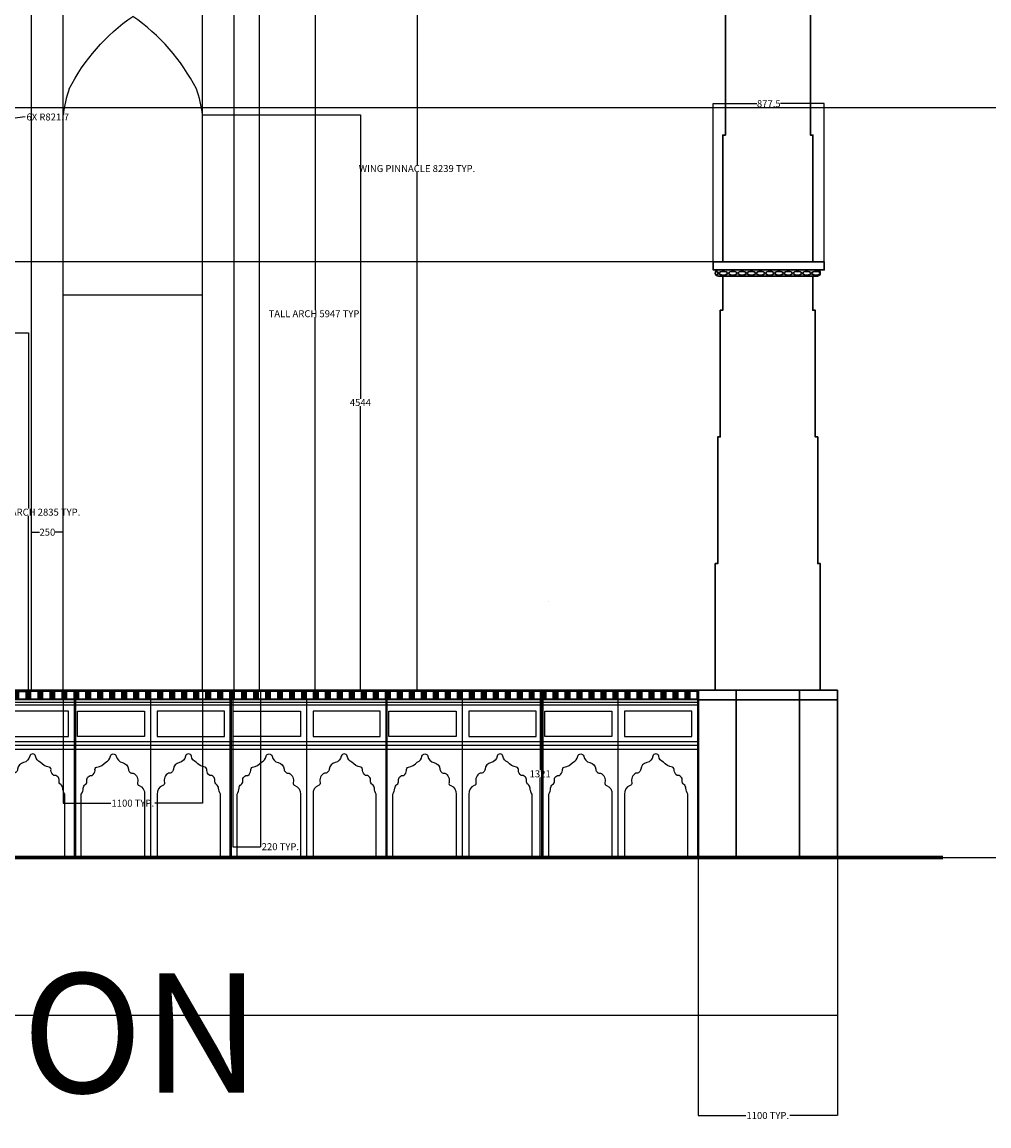
# Model space of a CAD drawing. Units: millimetres. Extents: x 8570 to 49085, y 3782 to 24863.
# Tile 8 of 15: x 27529 to 35169, y 3782 to 12499. Entities that reach past the tile are written whole.
import ezdxf

# ---------------------------------------------------------------- set-up
doc = ezdxf.new("R2010")
doc.units = ezdxf.units.MM
doc.header["$MEASUREMENT"] = 0
doc.header["$PDMODE"] = 3
for name, color, linetype, lineweight in [('A-ANNO-DIMS', 2, 'Continuous', 18), ('A-ANNO-TEXT', 7, 'Continuous', 25), ('A-ELEV-ARCH', 7, 'Continuous', 25), ('A-ELEV-GRND', 7, 'Continuous', 35), ('A-ELEV-MNRT', 7, 'Continuous', 30), ('A-ELEV-PATT', 252, 'Continuous', 13), ('A-ELEV-PIER', 7, 'Continuous', 25), ('A-ELEV-PLIN', 7, 'Continuous', 25)]:
    doc.layers.add(name, color=color, linetype=linetype, lineweight=lineweight)
doc.styles.get("Standard").update_dxf_attribs({"font": 'arial.ttf'})
doc.dimstyles.get("Standard").update_dxf_attribs({"dimtxt": 55, "dimasz": 0.18, "dimexe": 0.18, "dimexo": 0.0625, "dimgap": 0.09, "dimtad": 0, "dimtih": 1, "dimtoh": 1, "dimdec": 0, "dimzin": 0, "dimdsep": 46, "dimtxsty": 'Standard', "dimcen": 0.09, "dimadec": 0, "dimazin": 0, "dimtfac": 1, "dimtdec": 0, "dimtofl": 0, "dimtmove": 0, "dimatfit": 3, "dimfxl": 1, "dimtolj": 1, "dimtzin": 0, "dimarcsym": 0})

# ---------------------------------------------------------------- blocks, each defined once
blk = doc.blocks.new('MINARET-ELEV')
h = blk.add_hatch(color=256)
h.dxf.hatch_style = 1
edge = h.paths.add_edge_path()
edge.add_arc((788.1, 7879), 96, 347.52389, 357.31225, ccw=False)
edge.add_ellipse((859.2, 7847.7), major_axis=(31.8, 0), ratio=0.472441, start_angle=385.01443, end_angle=315.51296)
edge.add_arc((788.1, 7879), 96, 325.26025, 332.17741, ccw=False)
edge.add_line((867, 7824.3), (235, 7824.3))
edge.add_arc((313.9, 7879), 96, 182.68775, 214.73975, ccw=False)
edge.add_line((218, 7874.5), (884, 7874.5))
edge = h.paths.add_edge_path(flags=16)
edge.add_ellipse((494.2, 7847.7), major_axis=(31.8, 0), ratio=0.472441, start_angle=0, end_angle=360, ccw=False)
edge = h.paths.add_edge_path(flags=16)
edge.add_ellipse((567.2, 7847.7), major_axis=(31.8, 0), ratio=0.472441, start_angle=0, end_angle=360, ccw=False)
edge = h.paths.add_edge_path(flags=16)
edge.add_ellipse((421.2, 7847.7), major_axis=(31.8, 0), ratio=0.472441, start_angle=0, end_angle=360, ccw=False)
edge = h.paths.add_edge_path(flags=16)
edge.add_ellipse((640.2, 7847.7), major_axis=(31.8, 0), ratio=0.472441, start_angle=0, end_angle=360, ccw=False)
edge = h.paths.add_edge_path(flags=16)
edge.add_ellipse((348.2, 7847.7), major_axis=(31.8, 0), ratio=0.472441, start_angle=0, end_angle=360, ccw=False)
edge = h.paths.add_edge_path(flags=16)
edge.add_ellipse((713.2, 7847.7), major_axis=(31.8, 0), ratio=0.472441, start_angle=0, end_angle=360, ccw=False)
edge = h.paths.add_edge_path(flags=16)
edge.add_ellipse((275.2, 7847.7), major_axis=(31.8, 0), ratio=0.472441, start_angle=0, end_angle=360, ccw=False)
edge = h.paths.add_edge_path(flags=16)
edge.add_ellipse((786.2, 7847.7), major_axis=(31.8, 0), ratio=0.472441, start_angle=0, end_angle=360, ccw=False)
h = blk.add_hatch(color=256)
h.dxf.hatch_style = 1
edge = h.paths.add_edge_path()
edge.add_arc((940, 4615.3), 25, 270, 450, ccw=False)
edge.add_line((940, 4590.3), (160, 4590.3))
edge.add_arc((160, 4615.3), 25, 217.6761, 270, ccw=False)
edge.add_ellipse((127.2, 4613.7), major_axis=(31.8, 0), ratio=0.472441, start_angle=313.43175, end_angle=411.74889)
edge.add_arc((160, 4615.3), 25, 450, 510.08055, ccw=False)
edge.add_line((160, 4640.3), (940, 4640.3))
edge = h.paths.add_edge_path(flags=16)
edge.add_ellipse((347.2, 4613.7), major_axis=(31.8, 0), ratio=0.472441, start_angle=0, end_angle=360, ccw=False)
edge = h.paths.add_edge_path(flags=16)
edge.add_ellipse((420.2, 4613.7), major_axis=(31.8, 0), ratio=0.472441, start_angle=0, end_angle=360, ccw=False)
edge = h.paths.add_edge_path(flags=16)
edge.add_ellipse((274.2, 4613.7), major_axis=(31.8, 0), ratio=0.472441, start_angle=0, end_angle=360, ccw=False)
edge = h.paths.add_edge_path(flags=16)
edge.add_ellipse((493.2, 4613.7), major_axis=(31.8, 0), ratio=0.472441, start_angle=0, end_angle=360, ccw=False)
edge = h.paths.add_edge_path(flags=16)
edge.add_ellipse((198.8, 4613.7), major_axis=(31.8, 0), ratio=0.472441, start_angle=0, end_angle=360, ccw=False)
edge = h.paths.add_edge_path(flags=16)
edge.add_ellipse((566.2, 4613.7), major_axis=(31.8, 0), ratio=0.472441, start_angle=0, end_angle=360, ccw=False)
edge = h.paths.add_edge_path(flags=16)
edge.add_ellipse((639.2, 4613.7), major_axis=(31.8, 0), ratio=0.472441, start_angle=0, end_angle=360, ccw=False)
edge = h.paths.add_edge_path(flags=16)
edge.add_ellipse((712.2, 4613.7), major_axis=(31.8, 0), ratio=0.472441, start_angle=0, end_angle=360, ccw=False)
edge = h.paths.add_edge_path(flags=16)
edge.add_ellipse((785.2, 4613.7), major_axis=(31.8, 0), ratio=0.472441, start_angle=0, end_angle=360, ccw=False)
edge = h.paths.add_edge_path(flags=16)
edge.add_ellipse((858.2, 4613.7), major_axis=(31.8, 0), ratio=0.472441, start_angle=0, end_angle=360, ccw=False)
edge = h.paths.add_edge_path(flags=16)
edge.add_ellipse((931.2, 4613.7), major_axis=(31.8, 0), ratio=0.472441, start_angle=0, end_angle=360, ccw=False)
for p, q in [((851, 12922), (257.5, 12922)), ((257.5, 12922), (257.5, 12872)), ((851, 12922), (851, 12872)), ((851, 12897), (257.5, 12897)), ((851, 12872), (257.5, 12872)), ((298, 12162), (298, 12872)), ((556.7, 12843), (552, 12843)), ((815.5, 12162), (815.5, 12872)), ((348, 12162), (348, 12766.4)), ((423, 12162), (423, 12760.1)), ((690.5, 12162), (690.5, 12757.3)), ((765.5, 12162), (765.5, 12770.9)), ((815.5, 12162), (298, 12162)), ((807, 11939), (295, 11939)), ((867, 7824.3), (235, 7824.3)), ((867, 7824.3), (235, 7824.3)), ((160, 4590.3), (940, 4590.3)), ((165, 4590.3), (935, 4590.3)), ((905, 4590.3), (195, 4590.3)), ((300, 0), (300, 1321)), ((800, 0), (800, 1321)), ((1100, 0), (1100, 1321))]:
    blk.add_line(p, q)
blk.add_lwpolyline([(512, 13519.5, -0.216309), (551.3, 13585.8, -0.244698), (591, 13509.3, -0.244698)], format="xyb")
for points in [[(554, 13300, -0.140093), (458.9, 13405.9, -0.184272)], [(554, 13300, 0.140093), (646.7, 13408, 0.184272)]]:
    blk.add_lwpolyline(points, format="xyb", close=True)
for points in [[(815.5, 12072.5), (298, 12072.5), (298, 12162), (815.5, 12162)], [(898, 12072.5), (220.5, 12072.5), (220.5, 11989.2), (898, 11989.2)], [(948, 7939), (170.5, 7939), (170.5, 7874.5), (948, 7874.5)], [(997, 4705), (119.5, 4705), (119.5, 4640.5), (997, 4640.5)]]:
    blk.add_lwpolyline(points, close=True)
for points in [[(235, 7939), (235, 8939), (255, 8939), (255, 9939), (275, 9939), (275, 10939), (295, 10939), (295, 11939)], [(867, 7939), (867, 8939), (847, 8939), (847, 9939), (827, 9939), (827, 10939), (807, 10939), (807, 11939)], [(195, 4705), (195, 5705), (215, 5705), (215, 6705), (235, 6705), (235, 7824.3)], [(907, 4705), (907, 5705), (887, 5705), (887, 6705), (867, 6705), (867, 7824.3)], [(135, 1321), (135, 2321), (155, 2321), (155, 3321), (175, 3321), (175, 4321), (195, 4321), (195, 4590.3)], [(965, 1321), (965, 2321), (945, 2321), (945, 3321), (925, 3321), (925, 4321), (905, 4321), (905, 4590.3)], [(0, 1321), (1100, 1321)], [(0, 1246), (1100, 1246)]]:
    blk.add_lwpolyline(points)
for centre, radius in [((552, 13415.4), 63.1), ((554, 13261.5), 38.5)]:
    blk.add_circle(centre, radius)
for centre, radius, start, end in [((552, 13518.5), 40.1, 178.61203, 346.69346), ((554, 12961.3), 261.7, 351.36698, 188.63302), ((330.8, 12000.6), 71.3, 189.21146, 239.80255), ((759.2, 12000.8), 78.1, 307.68318, 351.42034), ((313.9, 7879), 96, 182.68775, 214.73975), ((788.1, 7879), 96, 325.26025, 357.31225), ((160, 4615.3), 25, 90, 270), ((940, 4615.3), 25, 270, 90)]:
    blk.add_arc(centre, radius, start, end)
at = {"extrusion": (0, 0, -1)}
for centre, start_param, end_param in [((275.2, 11962.4), -1.939365, 1.327018), ((348.2, 11962.4), -6.283185, 0), ((421.2, 11962.4), -6.283185, 0), ((494.2, 11962.4), -6.283185, 0), ((567.2, 11962.4), -6.283185, 0), ((640.2, 11962.4), -6.283185, 0), ((713.2, 11962.4), -6.283185, 0), ((786.2, 11962.4), -6.283185, 0), ((275.2, 7847.7), -6.283185, 0), ((348.2, 7847.7), -6.283185, 0), ((421.2, 7847.7), -6.283185, 0), ((494.2, 7847.7), -6.283185, 0), ((567.2, 7847.7), -6.283185, 0), ((640.2, 7847.7), -6.283185, 0), ((713.2, 7847.7), -6.283185, 0), ((786.2, 7847.7), -6.283185, 0), ((859.2, 7847.7), -5.160703, -0.779193), ((127.2, 4613.7), -1.214257, 1.150222), ((198.8, 4613.7), -6.283185, 0), ((274.2, 4613.7), -6.283185, 0), ((347.2, 4613.7), -6.283185, 0), ((420.2, 4613.7), -6.283185, 0), ((493.2, 4613.7), -6.283185, 0), ((566.2, 4613.7), -6.283185, 0), ((639.2, 4613.7), -6.283185, 0), ((712.2, 4613.7), -6.283185, 0), ((785.2, 4613.7), -6.283185, 0), ((858.2, 4613.7), -6.283185, 0), ((931.2, 4613.7), -6.283185, 0)]:
    blk.add_ellipse(centre, major_axis=(31.8, 0), ratio=0.472441, start_param=start_param, end_param=end_param, dxfattribs=at)
for points in [[(554.4, 12843), (553.6, 12843), (500.8, 12843), (391.9, 12680.1), (321.9, 12795.7), (298, 12872)], [(554.4, 12843), (555.2, 12843), (607.9, 12843), (716.8, 12680.1), (786.9, 12795.7), (815.5, 12872)]]:
    blk.add_open_spline(points, degree=3, knots=[136.061972, 136.061972, 136.061972, 136.061972, 139.000899, 330.944902, 463.724089, 463.724089, 463.724089, 463.724089])
blk = doc.blocks.new('PLINTH-PAIRED-BAY')
for p, q in [((623.5, 0), (623.5, 1246)), ((573.5, 0), (623.5, 0)), ((1173.5, 0), (1223.5, 0))]:
    blk.add_line(p, q)
for points in [[(0, 1309.5), (58.5, 1309.5), (58.5, 1253), (0, 1253)], [(94.7, 1309.5), (153.2, 1309.5), (153.2, 1253), (94.7, 1253)], [(189.5, 1309.5), (248, 1309.5), (248, 1253), (189.5, 1253)], [(284.2, 1309.5), (342.7, 1309.5), (342.7, 1253), (284.2, 1253)], [(378.9, 1309.5), (437.4, 1309.5), (437.4, 1253), (378.9, 1253)], [(473.7, 1309.5), (532.2, 1309.5), (532.2, 1253), (473.7, 1253)], [(568.4, 1309.5), (626.9, 1309.5), (626.9, 1253), (568.4, 1253)], [(663.2, 1309.5), (721.7, 1309.5), (721.7, 1253), (663.2, 1253)], [(757.9, 1309.5), (816.4, 1309.5), (816.4, 1253), (757.9, 1253)], [(852.6, 1309.5), (911.1, 1309.5), (911.1, 1253), (852.6, 1253)], [(947.4, 1309.5), (1005.9, 1309.5), (1005.9, 1253), (947.4, 1253)], [(1042.1, 1309.5), (1100.6, 1309.5), (1100.6, 1253), (1042.1, 1253)], [(1136.8, 1309.5), (1195.3, 1309.5), (1195.3, 1253), (1136.8, 1253)], [(42.5, 1156), (573.5, 1156), (573.5, 956), (42.5, 956)], [(1204.5, 1156), (673.5, 1156), (673.5, 956), (1204.5, 956)]]:
    blk.add_lwpolyline(points, close=True)
for points in [[(573.5, 500), (573.5, 0), (73.5, 0), (73.5, 500, 0.133896), (89, 547, -0.229833), (105, 576, 0.282739), (118.5, 607.5, -0.502693), (159, 648, 0.231145), (182, 687, -0.35399), (196, 714, 0.196071), (266.2, 753.9, 0.282071), (303.4, 799.6, -0.761042), (350.3, 800.8, 0.299945), (398, 749.1, -0.349607), (445.5, 697, 0.443472), (484, 666.5, -0.349941), (517, 591, 0.399043), (530.5, 568, -0.342474)], [(673.5, 500), (673.5, 0), (1173.5, 0), (1173.5, 500, -0.133896), (1158, 547, 0.229833), (1142, 576, -0.282739), (1128.5, 607.5, 0.502693), (1088, 648, -0.231145), (1065, 687, 0.35399), (1051, 714, -0.196071), (980.8, 753.9, -0.282071), (943.6, 799.6, 0.761042), (896.7, 800.8, -0.299945), (849, 749.1, 0.349607), (801.5, 697, -0.443472), (763, 666.5, 0.349941), (730, 591, -0.399043), (716.5, 568, 0.342474)]]:
    blk.add_lwpolyline(points, format="xyb", close=True)
blk = doc.blocks.new('PAVILION-EDGE-PINNACLE')
for p, q in [((10, 8089.5), (160, 8089.5)), ((10, 0), (10, 8069.5)), ((10, 8069.5), (160, 8069.5)), ((160, 0), (160, 8069.5)), ((160, 0), (160, 6876.5)), ((10, 0), (10, 6246.5))]:
    blk.add_line(p, q)
blk.add_lwpolyline([(101.6, 8204.8, 0.216309), (82.9, 8236.3, 0.244698), (64, 8200, 0.244698)], format="xyb")
for centre, radius, start, end in [((82.6, 8204.4), 19, 193.30654, 1.38797), ((153, 8055.1), 147, 117.52778, 166.47476), ((17, 8055.1), 147, 13.52524, 62.47222), ((10, 8079.5), 10, 90, 270), ((160, 8079.5), 10, 270, 90)]:
    blk.add_arc(centre, radius, start, end)
blk = doc.blocks.new('WING-END-PINNACLE')
for p, q in [((10, 8109.5), (210, 8109.5)), ((10, 8089.5), (210, 8089.5)), ((10, 0), (10, 8069.5)), ((10, 8069.5), (210, 8069.5)), ((210, 0), (210, 8069.5))]:
    blk.add_line(p, q)
blk.add_lwpolyline([(127.1, 8207.4, 0.216309), (108.4, 8238.9, 0.244698), (89.5, 8202.5, 0.244698)], format="xyb")
blk.add_circle((110.5, 8181), 7.02)
for centre, radius, start, end in [((108.1, 8206.9), 19, 193.30654, 1.38797), ((10, 8099.5), 10, 90, 270), ((-119.7, 8420.4), 336.9, 292.6494, 312.99463), ((340.2, 8421.1), 337.7, 227.0303, 247.32566), ((210, 8099.5), 10, 270, 90), ((10, 8079.5), 10, 90, 270), ((210, 8079.5), 10, 270, 90)]:
    blk.add_arc(centre, radius, start, end)
blk = doc.blocks.new('WING-TALL-ARCH')
for p, q in [((0, 5946.5), (1100, 5946.5)), ((0, 0), (0, 5946.5)), ((1100, 0), (1100, 5946.5)), ((0, 3123.2), (1100, 3123.2))]:
    blk.add_line(p, q)
for points in [[(47.9, 4748, -0.124525), (550, 5321.3, -0.124525)], [(1052.1, 4748, 0.124525), (550, 5321.3, 0.124525)]]:
    blk.add_lwpolyline(points, format="xyb")
for centre, start, end in [((817.4, 4459.8), 159.46554, 174.14569), ((282.6, 4459.8), 5.85431, 20.53446)]:
    blk.add_arc(centre, 821.7, start, end)
blk = doc.blocks.new('*D15')
at = {"layer": 'A-ANNO-DIMS', "color": 0, "lineweight": -2, "transparency": 16777216}
for p, q in [((33971.1, 19487.3), (36009.1, 19487.3)), ((36008.9, 19487.1), (36008.9, 12722.6)), ((36008.9, 5901.7), (36008.9, 12666.2)), ((33971.1, 5901.5), (36009.1, 5901.5))]:
    blk.add_line(p, q, dxfattribs=at)
at = {"layer": 'A-ANNO-DIMS', "color": 0, "transparency": 16777216}
for points in [[(36008.8, 19487.1), (36008.9, 19487.1), (36008.9, 19487.3)], [(36008.8, 5901.7), (36008.9, 5901.7), (36008.9, 5901.5)]]:
    blk.add_solid(points, dxfattribs=at)
at = {"layer": 'Defpoints', "color": 0, "transparency": 16777216}
for p in [(33971, 19487.3), (36008.9, 19487.3), (33971, 5901.5)]:
    blk.add_point(p, dxfattribs=at)
at = {"layer": 'A-ANNO-DIMS', "color": 0, "transparency": 16777216, "insert": (36008.9, 12694.4), "char_height": 55, "attachment_point": 5}
blk.add_mtext('\\A1;MINARET 13586 TYP.', dxfattribs=at)
blk = doc.blocks.new('*D16')
at = {"layer": 'A-ANNO-DIMS', "color": 0, "lineweight": -2, "transparency": 16777216}
for p, q in [((32871, 5901.4), (32871, 3863.4)), ((33971, 5901.4), (33971, 3863.4)), ((32871.2, 3863.6), (33246.9, 3863.6)), ((33970.8, 3863.6), (33595.1, 3863.6))]:
    blk.add_line(p, q, dxfattribs=at)
at = {"layer": 'A-ANNO-DIMS', "color": 0, "transparency": 16777216}
for points in [[(32871.2, 3863.7), (32871.2, 3863.6), (32871, 3863.6)], [(33970.8, 3863.7), (33970.8, 3863.6), (33971, 3863.6)]]:
    blk.add_solid(points, dxfattribs=at)
at = {"layer": 'Defpoints', "color": 0, "transparency": 16777216}
for p in [(32871, 5901.5), (33971, 5901.5), (33971, 3863.6)]:
    blk.add_point(p, dxfattribs=at)
at = {"layer": 'A-ANNO-DIMS', "color": 0, "transparency": 16777216, "insert": (33421, 3863.6), "char_height": 55, "attachment_point": 5}
blk.add_mtext('\\A1;1100 TYP.', dxfattribs=at)
blk = doc.blocks.new('*D23')
at = {"layer": 'A-ANNO-DIMS', "color": 0, "lineweight": -2, "transparency": 16777216}
for p, q in [((29414.1, 15461.4), (30650, 15461.4)), ((30649.8, 15461.2), (30649.8, 11370.5)), ((30649.8, 7222.7), (30649.8, 11313.4)), ((29414.1, 7222.5), (30650, 7222.5))]:
    blk.add_line(p, q, dxfattribs=at)
at = {"layer": 'A-ANNO-DIMS', "color": 0, "transparency": 16777216}
for points in [[(30649.8, 15461.2), (30649.9, 15461.2), (30649.8, 15461.4)], [(30649.8, 7222.7), (30649.9, 7222.7), (30649.8, 7222.5)]]:
    blk.add_solid(points, dxfattribs=at)
at = {"layer": 'Defpoints', "color": 0, "transparency": 16777216}
for p in [(29414, 15461.4), (30649.8, 15461.4), (29414, 7222.5)]:
    blk.add_point(p, dxfattribs=at)
at = {"layer": 'A-ANNO-DIMS', "color": 0, "transparency": 16777216, "insert": (30649.8, 11341.9), "char_height": 55, "attachment_point": 5}
blk.add_mtext('\\A1;WING PINNACLE 8239 TYP.', dxfattribs=at)
blk = doc.blocks.new('*D24')
at = {"layer": 'A-ANNO-DIMS', "color": 0, "lineweight": -2, "transparency": 16777216}
for p, q in [((29194, 7222.4), (29194, 5986.5)), ((29414, 7222.4), (29414, 5986.5)), ((29194.2, 5986.7), (29413.8, 5986.7)), ((29414, 5986.7), (29414.2, 5986.7))]:
    blk.add_line(p, q, dxfattribs=at)
at = {"layer": 'A-ANNO-DIMS', "color": 0, "transparency": 16777216}
for points in [[(29194.2, 5986.7), (29194.2, 5986.6), (29194, 5986.7)], [(29413.8, 5986.7), (29413.8, 5986.6), (29414, 5986.7)]]:
    blk.add_solid(points, dxfattribs=at)
at = {"layer": 'Defpoints', "color": 0, "transparency": 16777216}
for p in [(29194, 7222.5), (29414, 7222.5), (29414, 5986.7)]:
    blk.add_point(p, dxfattribs=at)
at = {"layer": 'A-ANNO-DIMS', "color": 0, "transparency": 16777216, "insert": (29570, 5986.7), "char_height": 55, "attachment_point": 5}
blk.add_mtext('\\A1;220 TYP.', dxfattribs=at)
blk = doc.blocks.new('*D29')
at = {"layer": 'A-ANNO-DIMS', "color": 0, "lineweight": -2, "transparency": 16777216}
for p, q in [((27154.1, 10045.8), (27579.4, 10045.8)), ((27579.2, 10045.6), (27579.2, 8656.9)), ((27579.2, 7211.2), (27579.2, 8599.8)), ((27154.1, 7211), (27579.4, 7211))]:
    blk.add_line(p, q, dxfattribs=at)
at = {"layer": 'A-ANNO-DIMS', "color": 0, "transparency": 16777216}
for points in [[(27579.2, 10045.6), (27579.2, 10045.6), (27579.2, 10045.8)], [(27579.2, 7211.2), (27579.2, 7211.2), (27579.2, 7211)]]:
    blk.add_solid(points, dxfattribs=at)
at = {"layer": 'Defpoints', "color": 0, "transparency": 16777216}
for p in [(27154, 10045.8), (27579.2, 10045.8), (27154, 7211)]:
    blk.add_point(p, dxfattribs=at)
at = {"layer": 'A-ANNO-DIMS', "color": 0, "transparency": 16777216, "insert": (27579.2, 8628.4), "char_height": 55, "attachment_point": 5}
blk.add_mtext('\\A1;LOWER ARCH 2835 TYP.', dxfattribs=at)
blk = doc.blocks.new('*D31')
at = {"layer": 'A-ANNO-DIMS', "color": 0, "lineweight": -2, "transparency": 16777216}
for p, q in [((28954.1, 13169), (29846.2, 13169)), ((29846, 13168.8), (29846, 10224.3)), ((29846, 7222.7), (29846, 10167.2)), ((28954.1, 7222.5), (29846.2, 7222.5))]:
    blk.add_line(p, q, dxfattribs=at)
at = {"layer": 'A-ANNO-DIMS', "color": 0, "transparency": 16777216}
for points in [[(29845.9, 13168.8), (29846, 13168.8), (29846, 13169)], [(29845.9, 7222.7), (29846, 7222.7), (29846, 7222.5)]]:
    blk.add_solid(points, dxfattribs=at)
at = {"layer": 'Defpoints', "color": 0, "transparency": 16777216}
for p in [(28954, 13169), (29846, 13169), (28954, 7222.5)]:
    blk.add_point(p, dxfattribs=at)
at = {"layer": 'A-ANNO-DIMS', "color": 0, "transparency": 16777216, "insert": (29846, 10195.7), "char_height": 55, "attachment_point": 5}
blk.add_mtext('\\A1;TALL ARCH 5947 TYP.', dxfattribs=at)
blk = doc.blocks.new('*D32')
at = {"layer": 'A-ANNO-DIMS', "color": 0, "lineweight": -2, "transparency": 16777216}
for p, q in [((27854, 7222.4), (27854, 6330.3)), ((28954, 7222.4), (28954, 6330.3)), ((27854.2, 6330.5), (28229.9, 6330.5)), ((28953.8, 6330.5), (28578.1, 6330.5))]:
    blk.add_line(p, q, dxfattribs=at)
at = {"layer": 'A-ANNO-DIMS', "color": 0, "transparency": 16777216}
for points in [[(27854.2, 6330.6), (27854.2, 6330.5), (27854, 6330.5)], [(28953.8, 6330.6), (28953.8, 6330.5), (28954, 6330.5)]]:
    blk.add_solid(points, dxfattribs=at)
at = {"layer": 'Defpoints', "color": 0, "transparency": 16777216}
for p in [(27854, 7222.5), (28954, 7222.5), (28954, 6330.5)]:
    blk.add_point(p, dxfattribs=at)
at = {"layer": 'A-ANNO-DIMS', "color": 0, "transparency": 16777216, "insert": (28404, 6330.5), "char_height": 55, "attachment_point": 5}
blk.add_mtext('\\A1;1100 TYP.', dxfattribs=at)
blk = doc.blocks.new('*D43')
at = {"layer": 'A-ANNO-DIMS', "color": 0, "lineweight": -2, "transparency": 16777216}
for p, q in [((10844, 5901.4), (10844, 4653.3)), ((33971, 5901.4), (33971, 4653.3)), ((10844.2, 4653.5), (22303.5, 4653.5)), ((33970.8, 4653.5), (22511.5, 4653.5))]:
    blk.add_line(p, q, dxfattribs=at)
at = {"layer": 'A-ANNO-DIMS', "color": 0, "transparency": 16777216}
for points in [[(10844.2, 4653.5), (10844.2, 4653.5), (10844, 4653.5)], [(33970.8, 4653.5), (33970.8, 4653.5), (33971, 4653.5)]]:
    blk.add_solid(points, dxfattribs=at)
at = {"layer": 'Defpoints', "color": 0, "transparency": 16777216}
for p in [(10844, 5901.5), (33971, 5901.5), (33971, 4653.5)]:
    blk.add_point(p, dxfattribs=at)
at = {"layer": 'A-ANNO-DIMS', "color": 0, "transparency": 16777216, "insert": (22407.5, 4653.5), "char_height": 55, "attachment_point": 5}
blk.add_mtext('\\A1;23127', dxfattribs=at)
blk = doc.blocks.new('*D50')
at = {"layer": 'A-ANNO-DIMS', "color": 0, "lineweight": -2, "transparency": 16777216}
for p, q in [((22407.6, 13259), (36055.2, 13259)), ((36055, 13258.8), (36055, 12570.2)), ((36055, 11825.2), (36055, 12513.8)), ((24254.1, 11825), (36055.2, 11825))]:
    blk.add_line(p, q, dxfattribs=at)
at = {"layer": 'A-ANNO-DIMS', "color": 0, "transparency": 16777216}
for points in [[(36055, 13258.8), (36055, 13258.8), (36055, 13259)], [(36055, 11825.2), (36055, 11825.2), (36055, 11825)]]:
    blk.add_solid(points, dxfattribs=at)
at = {"layer": 'Defpoints', "color": 0, "transparency": 16777216}
for p in [(22407.5, 13259), (36055, 13259), (24254, 11825)]:
    blk.add_point(p, dxfattribs=at)
at = {"layer": 'A-ANNO-DIMS', "color": 0, "transparency": 16777216, "insert": (36055, 12542), "char_height": 55, "attachment_point": 5}
blk.add_mtext('\\A1;1434', dxfattribs=at)
blk = doc.blocks.new('*D58')
at = {"layer": 'A-ANNO-DIMS', "color": 0, "lineweight": -2, "transparency": 16777216}
for p, q in [((32870.9, 7222.5), (31622.8, 7222.5)), ((31623, 7222.3), (31623, 6590.2)), ((31623, 5901.7), (31623, 6533.8)), ((32870.9, 5901.5), (31622.8, 5901.5))]:
    blk.add_line(p, q, dxfattribs=at)
at = {"layer": 'A-ANNO-DIMS', "color": 0, "transparency": 16777216}
for points in [[(31623, 7222.3), (31623, 7222.3), (31623, 7222.5)], [(31623, 5901.7), (31623, 5901.7), (31623, 5901.5)]]:
    blk.add_solid(points, dxfattribs=at)
at = {"layer": 'Defpoints', "color": 0, "transparency": 16777216}
for p in [(31623, 7222.5), (32871, 7222.5), (32871, 5901.5)]:
    blk.add_point(p, dxfattribs=at)
at = {"layer": 'A-ANNO-DIMS', "color": 0, "transparency": 16777216, "insert": (31623, 6562), "char_height": 55, "attachment_point": 5}
blk.add_mtext('\\A1;1321', dxfattribs=at)
blk = doc.blocks.new('*D59')
at = {"layer": 'A-ANNO-DIMS', "color": 0, "lineweight": -2, "transparency": 16777216}
for p, q in [((32990.4, 10606.5), (8684.3, 10606.5)), ((8684.5, 10606.3), (8684.5, 8942.7)), ((8684.5, 7222.7), (8684.5, 8886.3)), ((32870.9, 7222.5), (8684.3, 7222.5))]:
    blk.add_line(p, q, dxfattribs=at)
at = {"layer": 'A-ANNO-DIMS', "color": 0, "transparency": 16777216}
for points in [[(8684.5, 10606.3), (8684.5, 10606.3), (8684.5, 10606.5)], [(8684.5, 7222.7), (8684.5, 7222.7), (8684.5, 7222.5)]]:
    blk.add_solid(points, dxfattribs=at)
at = {"layer": 'Defpoints', "color": 0, "transparency": 16777216}
for p in [(8684.5, 10606.5), (32990.5, 10606.5), (32871, 7222.5)]:
    blk.add_point(p, dxfattribs=at)
at = {"layer": 'A-ANNO-DIMS', "color": 0, "transparency": 16777216, "insert": (8684.5, 8914.5), "char_height": 55, "attachment_point": 5}
blk.add_mtext('\\A1;3384', dxfattribs=at)
blk = doc.blocks.new('*D60')
at = {"layer": 'A-ANNO-DIMS', "color": 0, "lineweight": -2, "transparency": 16777216}
for p, q in [((33041.4, 13840.5), (8684.3, 13840.5)), ((8684.5, 13840.3), (8684.5, 12251.7)), ((8684.5, 10606.7), (8684.5, 12195.3)), ((32990.4, 10606.5), (8684.3, 10606.5))]:
    blk.add_line(p, q, dxfattribs=at)
at = {"layer": 'A-ANNO-DIMS', "color": 0, "transparency": 16777216}
for points in [[(8684.5, 13840.3), (8684.5, 13840.3), (8684.5, 13840.5)], [(8684.5, 10606.7), (8684.5, 10606.7), (8684.5, 10606.5)]]:
    blk.add_solid(points, dxfattribs=at)
at = {"layer": 'Defpoints', "color": 0, "transparency": 16777216}
for p in [(8684.5, 13840.5), (33041.5, 13840.5), (32990.5, 10606.5)]:
    blk.add_point(p, dxfattribs=at)
at = {"layer": 'A-ANNO-DIMS', "color": 0, "transparency": 16777216, "insert": (8684.5, 12223.5), "char_height": 55, "attachment_point": 5}
blk.add_mtext('\\A1;3234', dxfattribs=at)
blk = doc.blocks.new('*D63')
at = {"layer": 'A-ANNO-DIMS', "color": 0, "lineweight": -2, "transparency": 16777216}
for p, q in [((32990.5, 10606.6), (32990.5, 11854.7)), ((32990.7, 11854.5), (33336.1, 11854.5)), ((33867.8, 11854.5), (33522.4, 11854.5)), ((33868, 10606.6), (33868, 11854.7))]:
    blk.add_line(p, q, dxfattribs=at)
at = {"layer": 'A-ANNO-DIMS', "color": 0, "transparency": 16777216}
for points in [[(32990.7, 11854.5), (32990.7, 11854.5), (32990.5, 11854.5)], [(33867.8, 11854.5), (33867.8, 11854.5), (33868, 11854.5)]]:
    blk.add_solid(points, dxfattribs=at)
at = {"layer": 'Defpoints', "color": 0, "transparency": 16777216}
for p in [(33868, 11854.5), (32990.5, 10606.5), (33868, 10606.5)]:
    blk.add_point(p, dxfattribs=at)
at = {"layer": 'A-ANNO-DIMS', "color": 0, "transparency": 16777216, "insert": (33429.2, 11854.5), "char_height": 55, "attachment_point": 5}
blk.add_mtext('\\A1;877.5', dxfattribs=at)
blk = doc.blocks.new('*D67')
at = {"layer": 'A-ANNO-DIMS', "color": 0, "lineweight": -2, "transparency": 16777216}
for p, q in [((28954.1, 11766.1), (30202.2, 11766.1)), ((30202, 11765.9), (30202, 9522.4)), ((30202, 7222.7), (30202, 9466.2)), ((28954.1, 7222.5), (30202.2, 7222.5))]:
    blk.add_line(p, q, dxfattribs=at)
at = {"layer": 'A-ANNO-DIMS', "color": 0, "transparency": 16777216}
for points in [[(30202, 11765.9), (30202, 11765.9), (30202, 11766.1)], [(30202, 7222.7), (30202, 7222.7), (30202, 7222.5)]]:
    blk.add_solid(points, dxfattribs=at)
at = {"layer": 'Defpoints', "color": 0, "transparency": 16777216}
for p in [(28954, 11766.1), (28954, 7222.5), (30202, 7222.5)]:
    blk.add_point(p, dxfattribs=at)
at = {"layer": 'A-ANNO-DIMS', "color": 0, "transparency": 16777216, "insert": (30202, 9494.3), "char_height": 55, "attachment_point": 5}
blk.add_mtext('\\A1;4544', dxfattribs=at)
blk = doc.blocks.new('*D71')
at = {"layer": 'A-ANNO-DIMS', "color": 0, "lineweight": -2, "transparency": 16777216}
for p, q in [((27604, 7222.6), (27604, 8470.7)), ((27604.2, 8470.5), (27667.8, 8470.5)), ((27853.8, 8470.5), (27790.2, 8470.5)), ((27854, 7222.6), (27854, 8470.7))]:
    blk.add_line(p, q, dxfattribs=at)
at = {"layer": 'A-ANNO-DIMS', "color": 0, "transparency": 16777216}
for points in [[(27604.2, 8470.5), (27604.2, 8470.5), (27604, 8470.5)], [(27853.8, 8470.5), (27853.8, 8470.5), (27854, 8470.5)]]:
    blk.add_solid(points, dxfattribs=at)
at = {"layer": 'Defpoints', "color": 0, "transparency": 16777216}
for p in [(27854, 8470.5), (27604, 7222.5), (27854, 7222.5)]:
    blk.add_point(p, dxfattribs=at)
at = {"layer": 'A-ANNO-DIMS', "color": 0, "transparency": 16777216, "insert": (27729, 8470.5), "char_height": 55, "attachment_point": 5}
blk.add_mtext('\\A1;250', dxfattribs=at)
blk = doc.blocks.new('*D88')
at = {"layer": 'A-ANNO-DIMS', "color": 0, "lineweight": -2, "transparency": 16777216}
for p, q in [((27554, 11749.3), (27065.2, 11686.3)), ((26249.9, 11581.3), (26250.1, 11581.3)), ((26250, 11581.2), (26250, 11581.4))]:
    blk.add_line(p, q, dxfattribs=at)
at = {"layer": 'A-ANNO-DIMS', "color": 0, "transparency": 16777216}
blk.add_solid([(27065.2, 11686.3), (27065.2, 11686.3), (27065, 11686.3)], dxfattribs=at)
at = {"layer": 'Defpoints', "color": 0, "transparency": 16777216}
for p in [(27065, 11686.3), (26250, 11581.3)]:
    blk.add_point(p, dxfattribs=at)
at = {"layer": 'A-ANNO-DIMS', "color": 0, "transparency": 16777216, "insert": (27732.4, 11749.3), "char_height": 55, "attachment_point": 5}
blk.add_mtext('\\A1;6X R821.7', dxfattribs=at)
blk = doc.blocks.new('*D95')
at = {"layer": 'A-ANNO-DIMS', "color": 0, "lineweight": -2, "transparency": 16777216}
for p, q in [((48826.8, 12322.2), (42401, 10673.8)), ((31690.9, 7926.2), (31691.1, 7926.2)), ((31691, 7926.2), (31691, 7926.3))]:
    blk.add_line(p, q, dxfattribs=at)
at = {"layer": 'A-ANNO-DIMS', "color": 0, "transparency": 16777216}
blk.add_solid([(42401, 10673.8), (42401, 10673.7), (42400.9, 10673.7)], dxfattribs=at)
at = {"layer": 'Defpoints', "color": 0, "transparency": 16777216}
for p in [(42400.9, 10673.7), (31691, 7926.2)]:
    blk.add_point(p, dxfattribs=at)
at = {"layer": 'A-ANNO-DIMS', "color": 0, "transparency": 16777216, "insert": (48956.7, 12322.2), "char_height": 55, "attachment_point": 5}
blk.add_mtext('\\A1;R11057', dxfattribs=at)

msp = doc.modelspace()

# ---------------------------------------------------------------- hatches: boundary and pattern name
at = {"layer": 'A-ELEV-PATT'}
h = msp.add_hatch(dxfattribs=at)
h.set_pattern_fill('ANSI31', color=256)
h.set_pattern_definition([(45, (13541, 0), (-0.0883883476, 0.0883883476), [])])
h.paths.add_polyline_path([(26716, 7222.5), (27947, 7222.5), (27947, 7147.5), (26716, 7147.5)])
h.paths.add_polyline_path([(27028.37, 7154.5), (27086.87, 7154.5), (27086.87, 7211), (27028.37, 7211)], flags=16)
h.paths.add_polyline_path([(26992.13, 7211), (26933.63, 7211), (26933.63, 7154.5), (26992.13, 7154.5)], flags=16)
h.paths.add_polyline_path([(27123.11, 7154.5), (27181.61, 7154.5), (27181.61, 7211), (27123.11, 7211)], flags=16)
h.paths.add_polyline_path([(26897.39, 7211), (26838.89, 7211), (26838.89, 7154.5), (26897.39, 7154.5)], flags=16)
h.paths.add_polyline_path([(27217.84, 7154.5), (27276.34, 7154.5), (27276.34, 7211), (27217.84, 7211)], flags=16)
h.paths.add_polyline_path([(26802.66, 7211), (26744.16, 7211), (26744.16, 7154.5), (26802.66, 7154.5)], flags=16)
h.paths.add_polyline_path([(27312.58, 7154.5), (27371.08, 7154.5), (27371.08, 7211), (27312.58, 7211)], flags=16)
h.paths.add_polyline_path([(27407.32, 7154.5), (27465.82, 7154.5), (27465.82, 7211), (27407.32, 7211)], flags=16)
h.paths.add_polyline_path([(27502.05, 7154.5), (27560.55, 7154.5), (27560.55, 7211), (27502.05, 7211)], flags=16)
h.paths.add_polyline_path([(27596.79, 7154.5), (27655.29, 7154.5), (27655.29, 7211), (27596.79, 7211)], flags=16)
h.paths.add_polyline_path([(27691.53, 7154.5), (27750.03, 7154.5), (27750.03, 7211), (27691.53, 7211)], flags=16)
h.paths.add_polyline_path([(27786.26, 7154.5), (27844.76, 7154.5), (27844.76, 7211), (27786.26, 7211)], flags=16)
h.paths.add_polyline_path([(27881, 7154.5), (27939.5, 7154.5), (27939.5, 7211), (27881, 7211)], flags=16)
h = msp.add_hatch(dxfattribs=at)
h.set_pattern_fill('ANSI31', color=256)
h.set_pattern_definition([(45, (14772, 0), (-0.0883883476, 0.0883883476), [])])
h.paths.add_polyline_path([(27947, 7222.5), (29178, 7222.5), (29178, 7147.5), (27947, 7147.5)])
h.paths.add_polyline_path([(28259.37, 7154.5), (28317.87, 7154.5), (28317.87, 7211), (28259.37, 7211)], flags=16)
h.paths.add_polyline_path([(28223.13, 7211), (28164.63, 7211), (28164.63, 7154.5), (28223.13, 7154.5)], flags=16)
h.paths.add_polyline_path([(28354.11, 7154.5), (28412.61, 7154.5), (28412.61, 7211), (28354.11, 7211)], flags=16)
h.paths.add_polyline_path([(28128.39, 7211), (28069.89, 7211), (28069.89, 7154.5), (28128.39, 7154.5)], flags=16)
h.paths.add_polyline_path([(28448.84, 7154.5), (28507.34, 7154.5), (28507.34, 7211), (28448.84, 7211)], flags=16)
h.paths.add_polyline_path([(28033.66, 7211), (27975.16, 7211), (27975.16, 7154.5), (28033.66, 7154.5)], flags=16)
h.paths.add_polyline_path([(28543.58, 7154.5), (28602.08, 7154.5), (28602.08, 7211), (28543.58, 7211)], flags=16)
h.paths.add_polyline_path([(28638.32, 7154.5), (28696.82, 7154.5), (28696.82, 7211), (28638.32, 7211)], flags=16)
h.paths.add_polyline_path([(28733.05, 7154.5), (28791.55, 7154.5), (28791.55, 7211), (28733.05, 7211)], flags=16)
h.paths.add_polyline_path([(28827.79, 7154.5), (28886.29, 7154.5), (28886.29, 7211), (28827.79, 7211)], flags=16)
h.paths.add_polyline_path([(28922.53, 7154.5), (28981.03, 7154.5), (28981.03, 7211), (28922.53, 7211)], flags=16)
h.paths.add_polyline_path([(29017.26, 7154.5), (29075.76, 7154.5), (29075.76, 7211), (29017.26, 7211)], flags=16)
h.paths.add_polyline_path([(29112, 7154.5), (29170.5, 7154.5), (29170.5, 7211), (29112, 7211)], flags=16)
h = msp.add_hatch(dxfattribs=at)
h.set_pattern_fill('ANSI31', color=256)
h.set_pattern_definition([(45, (16003, 0), (-0.0883883476, 0.0883883476), [])])
h.paths.add_polyline_path([(29178, 7222.5), (30409, 7222.5), (30409, 7147.5), (29178, 7147.5)])
h.paths.add_polyline_path([(29490.37, 7154.5), (29548.87, 7154.5), (29548.87, 7211), (29490.37, 7211)], flags=16)
h.paths.add_polyline_path([(29454.13, 7211), (29395.63, 7211), (29395.63, 7154.5), (29454.13, 7154.5)], flags=16)
h.paths.add_polyline_path([(29585.11, 7154.5), (29643.61, 7154.5), (29643.61, 7211), (29585.11, 7211)], flags=16)
h.paths.add_polyline_path([(29359.39, 7211), (29300.89, 7211), (29300.89, 7154.5), (29359.39, 7154.5)], flags=16)
h.paths.add_polyline_path([(29679.84, 7154.5), (29738.34, 7154.5), (29738.34, 7211), (29679.84, 7211)], flags=16)
h.paths.add_polyline_path([(29264.66, 7211), (29206.16, 7211), (29206.16, 7154.5), (29264.66, 7154.5)], flags=16)
h.paths.add_polyline_path([(29774.58, 7154.5), (29833.08, 7154.5), (29833.08, 7211), (29774.58, 7211)], flags=16)
h.paths.add_polyline_path([(29869.32, 7154.5), (29927.82, 7154.5), (29927.82, 7211), (29869.32, 7211)], flags=16)
h.paths.add_polyline_path([(29964.05, 7154.5), (30022.55, 7154.5), (30022.55, 7211), (29964.05, 7211)], flags=16)
h.paths.add_polyline_path([(30058.79, 7154.5), (30117.29, 7154.5), (30117.29, 7211), (30058.79, 7211)], flags=16)
h.paths.add_polyline_path([(30153.53, 7154.5), (30212.03, 7154.5), (30212.03, 7211), (30153.53, 7211)], flags=16)
h.paths.add_polyline_path([(30248.26, 7154.5), (30306.76, 7154.5), (30306.76, 7211), (30248.26, 7211)], flags=16)
h.paths.add_polyline_path([(30343, 7154.5), (30401.5, 7154.5), (30401.5, 7211), (30343, 7211)], flags=16)
h = msp.add_hatch(dxfattribs=at)
h.set_pattern_fill('ANSI31', color=256)
h.set_pattern_definition([(45, (17234, 0), (-0.0883883476, 0.0883883476), [])])
h.paths.add_polyline_path([(30409, 7222.5), (31640, 7222.5), (31640, 7147.5), (30409, 7147.5)])
h.paths.add_polyline_path([(30721.37, 7154.5), (30779.87, 7154.5), (30779.87, 7211), (30721.37, 7211)], flags=16)
h.paths.add_polyline_path([(30685.13, 7211), (30626.63, 7211), (30626.63, 7154.5), (30685.13, 7154.5)], flags=16)
h.paths.add_polyline_path([(30816.11, 7154.5), (30874.61, 7154.5), (30874.61, 7211), (30816.11, 7211)], flags=16)
h.paths.add_polyline_path([(30590.39, 7211), (30531.89, 7211), (30531.89, 7154.5), (30590.39, 7154.5)], flags=16)
h.paths.add_polyline_path([(30910.84, 7154.5), (30969.34, 7154.5), (30969.34, 7211), (30910.84, 7211)], flags=16)
h.paths.add_polyline_path([(30495.66, 7211), (30437.16, 7211), (30437.16, 7154.5), (30495.66, 7154.5)], flags=16)
h.paths.add_polyline_path([(31005.58, 7154.5), (31064.08, 7154.5), (31064.08, 7211), (31005.58, 7211)], flags=16)
h.paths.add_polyline_path([(31100.32, 7154.5), (31158.82, 7154.5), (31158.82, 7211), (31100.32, 7211)], flags=16)
h.paths.add_polyline_path([(31195.05, 7154.5), (31253.55, 7154.5), (31253.55, 7211), (31195.05, 7211)], flags=16)
h.paths.add_polyline_path([(31289.79, 7154.5), (31348.29, 7154.5), (31348.29, 7211), (31289.79, 7211)], flags=16)
h.paths.add_polyline_path([(31384.53, 7154.5), (31443.03, 7154.5), (31443.03, 7211), (31384.53, 7211)], flags=16)
h.paths.add_polyline_path([(31479.26, 7154.5), (31537.76, 7154.5), (31537.76, 7211), (31479.26, 7211)], flags=16)
h.paths.add_polyline_path([(31574, 7154.5), (31632.5, 7154.5), (31632.5, 7211), (31574, 7211)], flags=16)
h = msp.add_hatch(dxfattribs=at)
h.set_pattern_fill('ANSI31', color=256)
h.set_pattern_definition([(45, (18465, 0), (-0.0883883476, 0.0883883476), [])])
h.paths.add_polyline_path([(31640, 7222.5), (32871, 7222.5), (32871, 7147.5), (31640, 7147.5)])
h.paths.add_polyline_path([(31952.37, 7154.5), (32010.87, 7154.5), (32010.87, 7211), (31952.37, 7211)], flags=16)
h.paths.add_polyline_path([(31916.13, 7211), (31857.63, 7211), (31857.63, 7154.5), (31916.13, 7154.5)], flags=16)
h.paths.add_polyline_path([(32047.11, 7154.5), (32105.61, 7154.5), (32105.61, 7211), (32047.11, 7211)], flags=16)
h.paths.add_polyline_path([(31821.39, 7211), (31762.89, 7211), (31762.89, 7154.5), (31821.39, 7154.5)], flags=16)
h.paths.add_polyline_path([(32141.84, 7154.5), (32200.34, 7154.5), (32200.34, 7211), (32141.84, 7211)], flags=16)
h.paths.add_polyline_path([(31726.66, 7211), (31668.16, 7211), (31668.16, 7154.5), (31726.66, 7154.5)], flags=16)
h.paths.add_polyline_path([(32236.58, 7154.5), (32295.08, 7154.5), (32295.08, 7211), (32236.58, 7211)], flags=16)
h.paths.add_polyline_path([(32331.32, 7154.5), (32389.82, 7154.5), (32389.82, 7211), (32331.32, 7211)], flags=16)
h.paths.add_polyline_path([(32426.05, 7154.5), (32484.55, 7154.5), (32484.55, 7211), (32426.05, 7211)], flags=16)
h.paths.add_polyline_path([(32520.79, 7154.5), (32579.29, 7154.5), (32579.29, 7211), (32520.79, 7211)], flags=16)
h.paths.add_polyline_path([(32615.53, 7154.5), (32674.03, 7154.5), (32674.03, 7211), (32615.53, 7211)], flags=16)
h.paths.add_polyline_path([(32710.26, 7154.5), (32768.76, 7154.5), (32768.76, 7211), (32710.26, 7211)], flags=16)
h.paths.add_polyline_path([(32805, 7154.5), (32863.5, 7154.5), (32863.5, 7211), (32805, 7211)], flags=16)

# ---------------------------------------------------------------- linework, layer by layer
at = {"layer": 'A-ELEV-GRND', "const_width": 30}
msp.add_lwpolyline([(9932.5, 5901.52), (34807, 5902)], dxfattribs=at)
at = {"layer": 'A-ELEV-PLIN'}
for p, q in [((27947, 5901.5), (27947, 7222.5)), ((30409, 5901.5), (30409, 7222.5))]:
    msp.add_line(p, q, dxfattribs=at)
at = {"layer": 'A-ELEV-PLIN', "const_width": 20}
for points in [[(27947, 5901.5), (27947, 7222.5)], [(29178, 5901.5), (29178, 7222.5)], [(30409, 5901.5), (30409, 7222.5)], [(31640, 5901.5), (31640, 7222.5)], [(32871, 5901.5), (32871, 7222.5)]]:
    msp.add_lwpolyline(points, dxfattribs=at)
at = {"layer": 'A-ELEV-PLIN'}
for points in [[(11944, 7127.5), (32871, 7127.5)], [(11944, 7107.5), (32871, 7107.5)], [(11944, 6817.5), (32871, 6817.5)], [(11944, 6787.5), (32871, 6787.5)], [(11944, 6757.5), (32871, 6757.5)]]:
    msp.add_lwpolyline(points, dxfattribs=at)

# ---------------------------------------------------------------- block references
at = {"layer": 'A-ELEV-ARCH'}
msp.add_blockref('WING-TALL-ARCH', (27854, 7222.5), dxfattribs=at)
at = {"layer": 'A-ELEV-MNRT'}
msp.add_blockref('MINARET-ELEV', (32871, 5901.5), dxfattribs=at)
at = {"layer": 'A-ELEV-PIER'}
for name, p in [('PAVILION-EDGE-PINNACLE', (27444, 7222.5)), ('WING-END-PINNACLE', (29194, 7222.5))]:
    msp.add_blockref(name, p, dxfattribs=at)
at = {"layer": 'A-ELEV-PLIN', "extrusion": (0, 0, -1), "zscale": -1}
for p in [(-27939.5, 5901.5), (-29170.5, 5901.5), (-30401.5, 5901.5), (-31632.5, 5901.5), (-32863.5, 5901.5)]:
    msp.add_blockref('PLINTH-PAIRED-BAY', p, dxfattribs=at)

# ---------------------------------------------------------------- texts
at = {"layer": 'A-ANNO-TEXT'}
msp.add_text('TAJ MAHAL ELEVATION', height=943, dxfattribs=at).set_placement((15583.5, 4043))

# ---------------------------------------------------------------- dimensions: what is measured, and where the dimension line sits
at = {"layer": 'A-ANNO-DIMS'}
for base, p1, p2, text, picture, middle in [((36008.87, 19487.32), (33971, 5901.5), (33971, 19487.32), 'MINARET <> TYP.', '*D15', (36008.87, 12694.41)), ((30649.83, 15461.36), (29414, 7222.5), (29414, 15461.36), 'WING PINNACLE <> TYP.', '*D23', (30649.83, 11341.93)), ((29845.975, 13169), (28954, 7222.5), (28954, 13169), 'TALL ARCH <> TYP.', '*D31', (29845.975, 10195.75)), ((27579.21, 10045.75), (27154, 7211), (27154, 10045.75), 'LOWER ARCH <> TYP.', '*D29', (27579.21, 8628.37))]:
    dim = msp.add_linear_dim(base=base, p1=p1, p2=p2, angle=90, text=text, dimstyle='Standard', override={"dimdec": 0, "dimlfac": 1, "dimrnd": 0, "dimzin": 0, "dimdsep": 46, "dimlunit": 2}, dxfattribs=at)
    dim.commit()
    dim.dimension.update_dxf_attribs({"geometry": picture, "text_midpoint": middle})
for base, p1, p2, angle, picture, middle in [((8684.5, 13840.5), (32990.5, 10606.5), (33041.5, 13840.5), 90, '*D60', (8684.5, 12223.5)), ((36055, 13259), (24254, 11825), (22407.5, 13259), 90, '*D50', (36055, 12542)), ((30202, 7222.5), (28954, 11766.11), (28954, 7222.5), 270, '*D67', (30202, 9494.31)), ((8684.5, 10606.5), (32871, 7222.5), (32990.5, 10606.5), 90, '*D59', (8684.5, 8914.5)), ((31623, 7222.5), (32871, 5901.5), (32871, 7222.5), 90, '*D58', (31623, 6562))]:
    dim = msp.add_linear_dim(base=base, p1=p1, p2=p2, angle=angle, dimstyle='Standard', override={"dimdec": 0, "dimlfac": 1, "dimrnd": 0, "dimzin": 0, "dimdsep": 46, "dimlunit": 2}, dxfattribs=at)
    dim.commit()
    dim.dimension.update_dxf_attribs({"geometry": picture, "text_midpoint": middle})
dim = msp.add_radius_dim(center=(31690.99, 7926.25), mpoint=(42400.86, 10673.71), dimstyle='Standard', override={"dimdec": 0, "dimlfac": 1, "dimrnd": 0, "dimzin": 0, "dimdsep": 46, "dimlunit": 2}, dxfattribs=at)
dim.commit()
dim.dimension.update_dxf_attribs({"geometry": '*D95', "text_midpoint": (48826.79, 12322.19), "dimtype": 164})
for base, p1, p2, override, picture, middle in [((33868, 11854.5), (32990.5, 10606.5), (33868, 10606.5), {"dimdec": 1, "dimlfac": 1, "dimrnd": 0, "dimzin": 0, "dimdsep": 46, "dimlunit": 2}, '*D63', (33429.25, 11854.5)), ((27854, 8470.5), (27604, 7222.5), (27854, 7222.5), {"dimdec": 0, "dimlfac": 1, "dimrnd": 0, "dimzin": 0, "dimdsep": 46, "dimlunit": 2}, '*D71', (27729, 8470.5)), ((33971, 4653.5), (10844, 5901.5), (33971, 5901.5), {"dimdec": 0, "dimlfac": 1, "dimrnd": 0, "dimzin": 0, "dimdsep": 46, "dimlunit": 2}, '*D43', (22407.5, 4653.5))]:
    dim = msp.add_linear_dim(base=base, p1=p1, p2=p2, dimstyle='Standard', override=override, dxfattribs=at)
    dim.commit()
    dim.dimension.update_dxf_attribs({"geometry": picture, "text_midpoint": middle})
dim = msp.add_radius_dim(center=(26249.99, 11581.31), mpoint=(27064.98, 11686.3), text='6X <>', dimstyle='Standard', override={"dimdec": 1, "dimlfac": 1, "dimrnd": 0, "dimzin": 0, "dimdsep": 46, "dimlunit": 2}, dxfattribs=at)
dim.commit()
dim.dimension.update_dxf_attribs({"geometry": '*D88', "text_midpoint": (27553.97, 11749.28), "dimtype": 164})
for base, p1, p2, picture, middle in [((28954, 6330.53), (27854, 7222.5), (28954, 7222.5), '*D32', (28404, 6330.53)), ((29414, 5986.67), (29194, 7222.5), (29414, 7222.5), '*D24', (29569.97, 5986.67)), ((33971, 3863.63), (32871, 5901.5), (33971, 5901.5), '*D16', (33421, 3863.63))]:
    dim = msp.add_linear_dim(base=base, p1=p1, p2=p2, text='<> TYP.', dimstyle='Standard', override={"dimdec": 0, "dimlfac": 1, "dimrnd": 0, "dimzin": 0, "dimdsep": 46, "dimlunit": 2}, dxfattribs=at)
    dim.commit()
    dim.dimension.update_dxf_attribs({"geometry": picture, "text_midpoint": middle})

doc.saveas('drawing.dxf')
